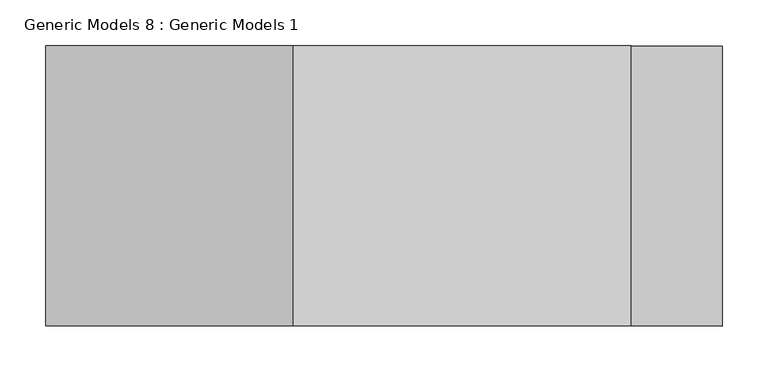
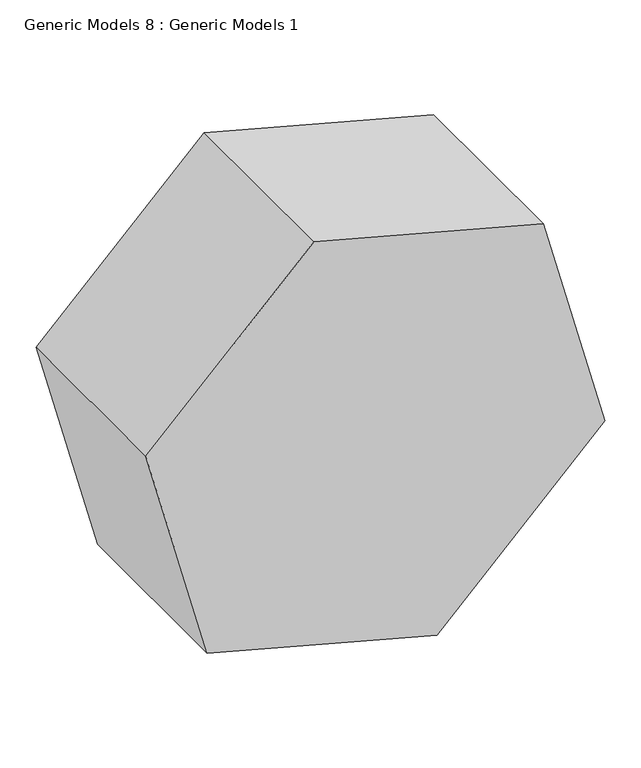
"""IFC4 building model written with IfcOpenShell, lengths in millimetres: proxy geometry, Generic Models 8 : Generic Models 1."""

from ifc_helpers import new_model, si_unit, frame, origin, place, context, project, spatial, polyline, outline, extrude, source, transform, mapped, element, save


def generic_models_8_generic_models_1_b8e4b7b0(model_context):
    return source(origin(), model_context, "Body", "SweptSolid", [
        extrude(outline(polyline([(904.7566299, -3548.6070438), (1003.366686, -3916.6247836), (733.9590024, -4186.0324672), (365.9412626, -4087.422411), (267.3312064, -3719.4046712), (536.73889, -3449.9969876), (904.7566299, -3548.6070438)])), frame((0.0, -9086.6225464, 0.0), z_axis=(0.0, 1.0, 0.0), x_axis=(0.0, 0.0, 1.0)), (0.0, 0.0, 1.0), 304.8),
    ])


if __name__ == "__main__":
    model = new_model("IFC4")
    model_context = context("Model", 3, world=origin())
    ifc_project = project(units=[si_unit("LENGTHUNIT", "METRE", prefix="MILLI")], contexts=[model_context])
    site = spatial("IfcSite", under=ifc_project)
    building = spatial("IfcBuilding", under=site)
    placement = place(None, origin())
    generic_models_8_generic_models_1_shape = generic_models_8_generic_models_1_b8e4b7b0(model_context)
    element("IfcBuildingElementProxy", 1, Name="Generic Models 8 : Generic Models 1", ObjectType="Generic Models 8 : Generic Models 1", at=placement, inside=building, context=model_context, shape_type="MappedRepresentation", body=[
        mapped(generic_models_8_generic_models_1_shape, transform((0.0, 0.0, 0.0), x_axis=(1.0, 0.0, 0.0), y_axis=(0.0, 1.0, 0.0), z_axis=(0.0, 0.0, 1.0))),
    ])
    save(model, "model.ifc")

# Revit data of these elements
# Element 1 (IfcBuildingElementProxy, "Generic Models 8 : Generic Models 1")
#   Materials on its faces: "Brick, Common"
# Materials
#   "Brick, Common": class "Masonry", colour RGB 170 98 104, transparency 0, Description = "Common brick", Cost = 0
